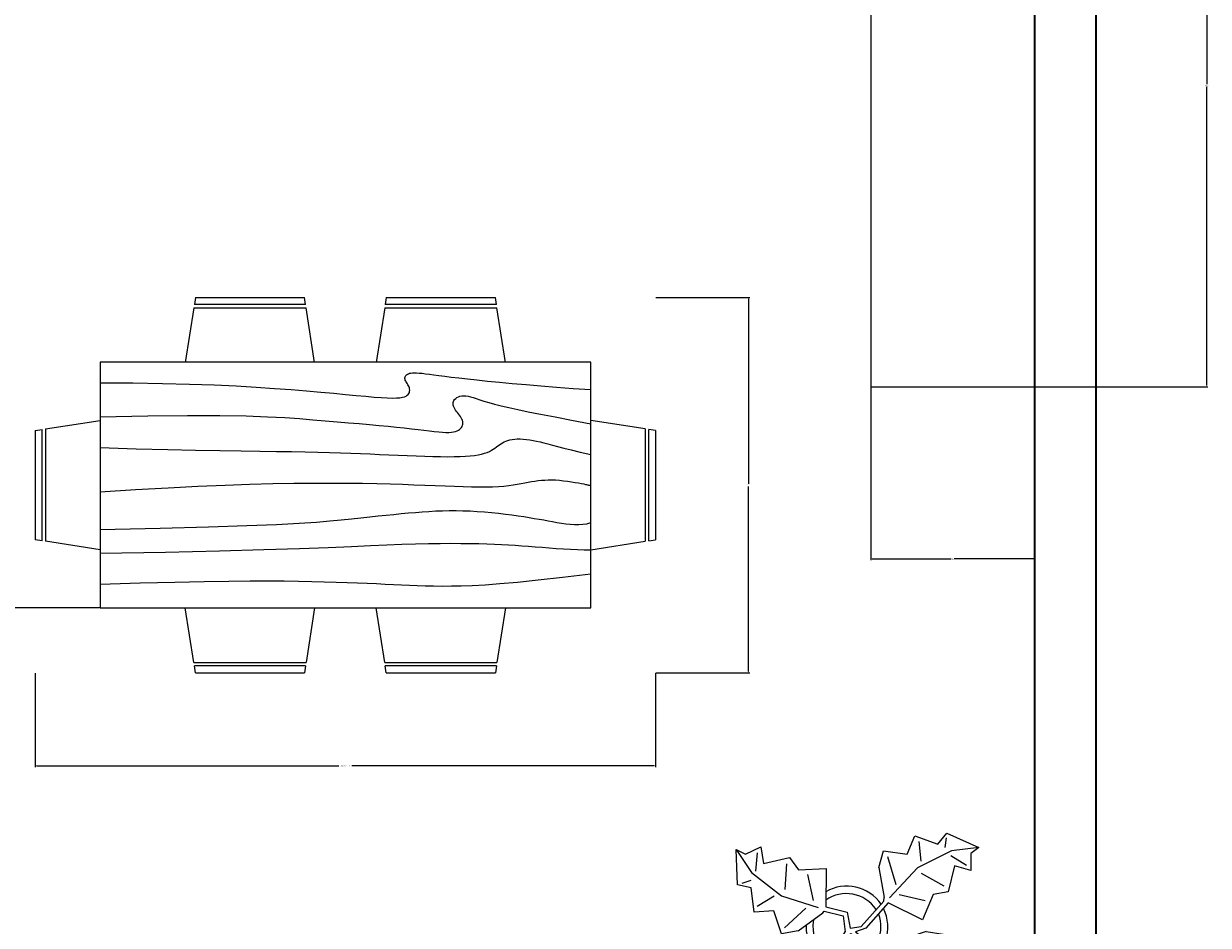
# Model space of a CAD drawing. Units: inches. Extents: x -1 to 436, y -13 to 497.
# Tile 3 of 4: x 227 to 400, y 183 to 315. Entities that reach past the tile are written whole.
import ezdxf

# ---------------------------------------------------------------- set-up
doc = ezdxf.new("R2010")
doc.units = ezdxf.units.IN
for name, color, linetype, lineweight in [('A-ANNO-DIMS', 2, 'Continuous', 18), ('A-FLOR-CASE', 8, 'Continuous', 25), ('A-FURN', 8, 'Continuous', 18), ('A-PLNT', 3, 'Continuous', 13), ('A-WALL', 7, 'Continuous', 35)]:
    doc.layers.add(name, color=color, linetype=linetype, lineweight=lineweight)
doc.styles.get("Standard").update_dxf_attribs({"font": 'arial.ttf'})
doc.dimstyles.get("Standard").update_dxf_attribs({"dimtxt": 0.18, "dimasz": 0.18, "dimexe": 0.18, "dimexo": 0.0625, "dimgap": 0.09, "dimtad": 0, "dimtih": 1, "dimtoh": 1, "dimdec": 4, "dimzin": 0, "dimdsep": 46, "dimtxsty": 'Standard', "dimcen": 0.09, "dimadec": 0, "dimazin": 0, "dimtfac": 1, "dimtdec": 4, "dimtofl": 0, "dimtmove": 0, "dimatfit": 3, "dimfxl": 1, "dimtolj": 1, "dimtzin": 0, "dimarcsym": 0})

# ---------------------------------------------------------------- blocks, each defined once
blk = doc.blocks.new('Dining Set - 36 x 72 in.')
for p, q in [((-22, 27.5), (-22.1562, 26.50042)), ((-5.8416, 26.5), (-22.1534, 26.5)), ((-22, 27.5), (-6, 27.5)), ((-5.8437, 26.49966), (-6, 27.5)), ((6, 27.5), (5.8438, 26.50042)), ((22.1584, 26.5), (5.8466, 26.5)), ((6, 27.5), (22, 27.5)), ((22.1563, 26.49966), (22, 27.5)), ((-22.2343, 26.00059), (-23.4847, 17.99762)), ((-22.2304, 26), (-5.7608, 26)), ((-4.5152, 17.99762), (-5.7655, 25.99926)), ((5.7657, 26.00059), (4.5153, 17.99762)), ((5.7696, 26), (22.2392, 26)), ((23.4848, 17.99762), (22.2345, 25.99926)), ((36, 18), (-36, 18)), ((-36, 18), (-36, -18)), ((36, -18), (36, 18)), ((-44.0006, 8.23428), (-35.9976, 9.48474)), ((44.0006, 8.23428), (35.9976, 9.48474)), ((-45.5, 8), (-44.5004, 8.15617)), ((-45.5, 8), (-45.5, -8)), ((-44.5, -8.15843), (-44.5, 8.15338)), ((-44, 8.23041), (-44, -8.23915)), ((44, 8.23041), (44, -8.23915)), ((44.5, -8.15843), (44.5, 8.15338)), ((45.5, 8), (44.5005, 8.15617)), ((45.5, 8), (45.5, -8)), ((-44.4997, -8.15631), (-45.5, -8)), ((-35.9976, -9.48476), (-43.9993, -8.2345)), ((35.9976, -9.48476), (43.9993, -8.2345)), ((44.4997, -8.15631), (45.5, -8)), ((-36, -18), (36, -18)), ((-22.2343, -26.0006), (-23.4847, -17.99762)), ((-4.5152, -17.99762), (-5.7655, -25.99928)), ((5.7657, -26.0006), (4.5153, -17.99762)), ((23.4848, -17.99762), (22.2345, -25.99928)), ((-22.2304, -26), (-5.7608, -26)), ((5.7696, -26), (22.2392, -26)), ((-22, -27.5), (-22.1562, -26.50044)), ((-5.8416, -26.5), (-22.1534, -26.5)), ((-22, -27.5), (-6, -27.5)), ((-5.8437, -26.49967), (-6, -27.5)), ((6, -27.5), (5.8438, -26.50044)), ((22.1584, -26.5), (5.8466, -26.5)), ((6, -27.5), (22, -27.5)), ((22.1563, -26.49967), (22, -27.5))]:
    blk.add_line(p, q)
for points in [[(-36, 15), (-31.1772, 14.97754), (-26.8079, 14.91406), (-22.8538, 14.81543), (-19.276, 14.6875), (-16.0362, 14.53613), (-13.0957, 14.36718), (-10.4159, 14.18652), (-7.9583, 14), (-5.6904, 13.81315), (-3.6035, 13.63021), (-1.6954, 13.45508), (0.0365, 13.29166), (1.5945, 13.14388), (2.9811, 13.01562), (4.1988, 12.9108), (5.25, 12.83333), (6.1393, 12.78613), (6.8802, 12.76823), (7.4883, 12.77767), (7.9792, 12.8125), (8.3685, 12.87077), (8.6719, 12.95052), (8.9049, 13.0498), (9.0833, 13.16666), (9.2205, 13.29899), (9.3216, 13.44401), (9.3895, 13.59879), (9.4271, 13.76041), (9.4373, 13.92594), (9.4232, 14.09245), (9.3875, 14.257), (9.3333, 14.41666), (9.2638, 14.56917), (9.1836, 14.71484), (9.0975, 14.85465), (9.0104, 14.98958), (8.9272, 15.1206), (8.8529, 15.2487), (8.7922, 15.37483), (8.75, 15.5), (8.7305, 15.62467), (8.7344, 15.74739), (8.7617, 15.86621), (8.8125, 15.97916), (8.8867, 16.08431), (8.9844, 16.17968), (9.1055, 16.26334), (9.25, 16.33333), (9.4189, 16.38802), (9.6172, 16.42708), (9.8506, 16.45052), (10.125, 16.45833), (10.4463, 16.45052), (10.8203, 16.42708), (11.2529, 16.38802), (11.75, 16.33333), (12.3184, 16.26318), (12.9694, 16.17838), (13.7151, 16.07991), (14.5677, 15.96875), (15.5395, 15.84586), (16.6426, 15.71224), (17.8893, 15.56884), (19.2917, 15.41666), (20.859, 15.25667), (22.5879, 15.08984), (24.4721, 14.91715), (26.5052, 14.73958), (28.6809, 14.5581), (30.9929, 14.3737), (33.4347, 14.18733), (36, 14)], [(-36, 10), (-28.9766, 10.14274), (-23.1725, 10.20442), (-18.4241, 10.19775), (-14.5677, 10.13541), (-11.4399, 10.03011), (-8.877, 9.89453), (-6.7154, 9.74137), (-4.7917, 9.58333), (-2.9698, 9.43082), (-1.2246, 9.28515), (0.4415, 9.14534), (2.026, 9.01041), (3.5266, 8.87939), (4.9408, 8.7513), (6.266, 8.62516), (7.5, 8.5), (8.6411, 8.37549), (9.6914, 8.2539), (10.6538, 8.13818), (11.5312, 8.03125), (12.3267, 7.93603), (13.043, 7.85547), (13.6831, 7.79248), (14.25, 7.75), (14.7471, 7.7303), (15.1797, 7.73307), (15.5537, 7.75732), (15.875, 7.80208), (16.1494, 7.86637), (16.3828, 7.94922), (16.5811, 8.04964), (16.75, 8.16666), (16.8944, 8.29915), (17.0143, 8.44531), (17.1089, 8.60319), (17.1771, 8.77083), (17.218, 8.94629), (17.2305, 9.1276), (17.2137, 9.31282), (17.1667, 9.5), (17.0895, 9.6875), (16.987, 9.875), (16.8649, 10.0625), (16.7292, 10.25), (16.5856, 10.4375), (16.4401, 10.625), (16.2985, 10.8125), (16.1667, 11), (16.05, 11.18733), (15.9518, 11.3737), (15.8752, 11.5581), (15.8229, 11.73958), (15.798, 11.91715), (15.8034, 12.08984), (15.842, 12.25667), (15.9167, 12.41666), (16.0295, 12.56836), (16.1784, 12.70833), (16.3605, 12.83268), (16.5729, 12.9375), (16.8127, 13.01888), (17.0768, 13.07291), (17.3625, 13.0957), (17.6667, 13.08333), (17.9894, 13.03312), (18.3418, 12.94726), (18.7382, 12.82918), (19.1927, 12.68229), (19.7195, 12.51001), (20.3327, 12.31575), (21.0465, 12.10294), (21.875, 11.875), (22.8357, 11.63354), (23.959, 11.37304), (25.2786, 11.08618), (26.8282, 10.76562), (28.6414, 10.40405), (30.752, 9.99414), (33.1936, 9.52856), (36, 9)], [(-36, 5.5), (-30.7157, 5.3348), (-26.069, 5.20963), (-21.9946, 5.11767), (-18.4271, 5.05208), (-15.3009, 5.00602), (-12.5508, 4.97265), (-10.1112, 4.94515), (-7.9167, 4.91666), (-5.909, 4.88167), (-4.0586, 4.83984), (-2.3429, 4.79215), (-0.7396, 4.73958), (0.7739, 4.6831), (2.22, 4.6237), (3.6213, 4.56233), (5, 4.5), (6.373, 4.43782), (7.7344, 4.3776), (9.0723, 4.32129), (10.375, 4.27083), (11.6309, 4.22819), (12.8281, 4.19531), (13.9551, 4.17415), (15, 4.16666), (15.954, 4.17448), (16.819, 4.19791), (17.6001, 4.23698), (18.3021, 4.29166), (18.9299, 4.36198), (19.4883, 4.44791), (19.9823, 4.54948), (20.4167, 4.66666), (20.7969, 4.79899), (21.1302, 4.94401), (21.4245, 5.09879), (21.6875, 5.26041), (21.9271, 5.42594), (22.1511, 5.59245), (22.3672, 5.757), (22.5834, 5.91666), (22.8065, 6.06868), (23.0404, 6.21093), (23.2879, 6.34147), (23.5521, 6.45833), (23.8358, 6.55957), (24.142, 6.64323), (24.4735, 6.70735), (24.8334, 6.75), (25.2235, 6.76969), (25.642, 6.76692), (26.0858, 6.74267), (26.5521, 6.69791), (27.0379, 6.63362), (27.5404, 6.55078), (28.0565, 6.45036), (28.5834, 6.33333), (29.1242, 6.19987), (29.7071, 6.04687), (30.3661, 5.87044), (31.1354, 5.66666), (32.0493, 5.43164), (33.142, 5.16146), (34.4475, 4.85221), (36, 4.5)], [(-36, -1), (-30.7915, -0.6591), (-26.0195, -0.38216), (-21.6519, -0.16284), (-17.6563, 0.00521), (-14.0005, 0.12833), (-10.6523, 0.21289), (-7.5796, 0.26522), (-4.75, 0.29166), (-2.134, 0.29793), (0.2878, 0.28711), (2.5317, 0.26163), (4.6146, 0.22396), (6.5529, 0.17651), (8.3633, 0.12174), (10.0623, 0.06209), (11.6667, 0), (13.1899, -0.06201), (14.6341, -0.1211), (15.9982, -0.17432), (17.2813, -0.21875), (18.4823, -0.25147), (19.6003, -0.26953), (20.6343, -0.27002), (21.5834, -0.25), (22.4481, -0.20768), (23.2357, -0.14584), (23.9549, -0.06836), (24.6146, 0.02083), (25.2235, 0.11784), (25.7904, 0.21875), (26.3241, 0.31966), (26.8334, 0.41666), (27.3265, 0.50618), (27.8099, 0.58593), (28.2894, 0.65397), (28.7709, 0.70833), (29.2601, 0.74707), (29.763, 0.76823), (30.2855, 0.76985), (30.8334, 0.75), (31.4088, 0.70784), (31.9994, 0.64713), (32.589, 0.57275), (33.1615, 0.48958), (33.7008, 0.4025), (34.1908, 0.3164), (34.6153, 0.23616), (34.9584, 0.16666), (35.2099, 0.11165), (35.3848, 0.07031), (35.504, 0.04069), (35.5886, 0.02083), (35.6594, 0.00879), (35.7377, 0.0026), (35.8442, 0.00032), (36, 0)], [(-36, -6.5), (-27.1843, -6.31267), (-20.084, -6.1263), (-14.469, -5.9419), (-10.1094, -5.76042), (-6.7752, -5.58285), (-4.2363, -5.41016), (-2.2629, -5.24333), (-0.625, -5.08334), (0.8708, -4.93099), (2.2715, -4.78646), (3.5872, -4.64974), (4.8281, -4.52084), (6.0046, -4.39974), (7.127, -4.28646), (8.2053, -4.18099), (9.25, -4.08334), (10.2705, -3.99382), (11.2734, -3.91407), (12.2647, -3.84603), (13.25, -3.79167), (14.2354, -3.75293), (15.2266, -3.73177), (16.2295, -3.73015), (17.25, -3.75), (18.2912, -3.79248), (19.3451, -3.85547), (20.4009, -3.93604), (21.4479, -4.03125), (22.4754, -4.13819), (23.4727, -4.25391), (24.4289, -4.37549), (25.3334, -4.5), (26.1785, -4.62492), (26.9694, -4.74935), (27.7145, -4.87281), (28.4219, -4.99479), (29.1, -5.11483), (29.7572, -5.23242), (30.4016, -5.34709), (31.0417, -5.45834), (31.6837, -5.56437), (32.3262, -5.65821), (32.9658, -5.73153), (33.599, -5.77604), (34.2224, -5.78345), (34.8327, -5.74545), (35.4264, -5.65373), (36, -5.5)], [(-36, -10), (-26.4022, -9.81299), (-18.4675, -9.62891), (-11.9839, -9.45069), (-6.7396, -9.28125), (-2.5226, -9.12354), (0.8789, -8.98047), (3.6769, -8.85498), (6.0833, -8.75), (8.2767, -8.66765), (10.3021, -8.60677), (12.1712, -8.56543), (13.8958, -8.54167), (15.4876, -8.53353), (16.9583, -8.53907), (18.3197, -8.55632), (19.5834, -8.58334), (20.7616, -8.61841), (21.8685, -8.66081), (22.9188, -8.71004), (23.9271, -8.76563), (24.9081, -8.82707), (25.8763, -8.89388), (26.8465, -8.96558), (27.8334, -9.04167), (28.8474, -9.12118), (29.8828, -9.20117), (30.93, -9.27824), (31.9792, -9.34896), (33.0205, -9.40991), (34.0443, -9.45768), (35.0407, -9.48885), (36, -9.5)], [(-36, -14.5), (-30.0881, -14.33513), (-25.0332, -14.21224), (-20.7312, -14.12647), (-17.0781, -14.07292), (-13.97, -14.04671), (-11.3027, -14.04297), (-8.9724, -14.05681), (-6.875, -14.08334), (-4.9224, -14.11833), (-3.0905, -14.16016), (-1.3709, -14.20785), (0.2448, -14.26042), (1.7647, -14.3169), (3.1973, -14.3763), (4.5507, -14.43767), (5.8333, -14.5), (7.0554, -14.5621), (8.235, -14.62175), (9.3922, -14.67652), (10.5469, -14.72396), (11.7192, -14.76164), (12.929, -14.78711), (14.1965, -14.79794), (15.5417, -14.79167), (16.9933, -14.76424), (18.6152, -14.70508), (20.4804, -14.60197), (22.6615, -14.44271), (25.2312, -14.21509), (28.2624, -13.9069), (31.8277, -13.50594), (36, -13)]]:
    blk.add_lwpolyline(points)
blk = doc.blocks.new('Plant - Rubber or Philodendron')
for p, q in [((13.3837, 12.301), (14.68, 13.9039)), ((14.68, 13.9039), (19.3848, 11.8146)), ((8.8871, 10.7908), (9.9809, 13.4933)), ((9.9809, 13.4933), (13.3837, 12.301)), ((10.5828, 12.6946), (10.8893, 9.7953)), ((14.5816, 13.2037), (14.3848, 11.8033)), ((-16.2005, 11.4774), (-13.9899, 8.1064)), ((-16.2005, 11.4774), (-14.8639, 10.7964)), ((-16.0159, 6.3329), (-16.2005, 11.4774)), ((-14.8639, 10.7964), (-12.6195, 11.8975)), ((-13.3174, 8.325), (-13.0735, 11.0065)), ((-12.6195, 11.8975), (-12.1909, 9.4345)), ((4.6914, 8.8812), (5.3859, 11.2828)), ((5.3859, 11.2828), (8.8871, 10.7908)), ((5.9878, 10.4842), (7.1971, 6.3869)), ((15.3859, 11.3055), (10.3916, 8.7942)), ((15.2875, 10.6053), (17.5907, 9.2105)), ((19.3848, 11.8146), (15.3859, 11.3055)), ((19.3848, 11.8146), (18.1868, 10.9119)), ((18.1868, 10.9119), (18.1925, 8.4119)), ((-12.1909, 9.4345), (-8.3829, 10.3)), ((-8.8369, 9.409), (-9.0894, 5.6095)), ((-8.3829, 10.3), (-7.0549, 8.501)), ((-7.0549, 8.501), (-3.0284, 8.6941)), ((-3.0284, 8.6941), (-3.0709, 3.1041)), ((4.6914, 8.8812), (5.5014, 4.4831)), ((10.3916, 8.7942), (6.2847, 4.4028)), ((15.7909, 9.1065), (14.8995, 5.3044)), ((18.1925, 8.4119), (15.7909, 9.1065)), ((-15.3434, 6.5514), (-13.9984, 6.9884)), ((-13.9899, 8.1064), (-9.5434, 4.7185)), ((-4.8529, 4.012), (-5.7184, 7.82)), ((14.2977, 6.1031), (10.9934, 7.9956)), ((-14.0069, 5.8704), (-16.0159, 6.3329)), ((-13.5868, 2.2894), (-14.0069, 5.8704)), ((14.8995, 5.3044), (12.7005, 4.8994)), ((-13.1329, 3.1804), (-10.6614, 4.727)), ((-9.5434, 4.7185), (-4.1917, 2.9888)), ((2.1141, 0.2298), (5.4346, 3.9146)), ((6.1032, 3.6844), (2.8262, -0.031)), ((5.4346, 3.9146), (5.5014, 4.4831)), ((11.1089, 1.1958), (6.1032, 3.6844)), ((7.7005, 4.8881), (11.5025, 3.9967)), ((12.7005, 4.8994), (11.1089, 1.1958)), ((-10.6784, 2.491), (-13.5868, 2.2894)), ((-9.5858, -0.8715), (-10.6784, 2.491)), ((-9.1318, 0.0195), (-5.9793, 2.9025)), ((-7.1228, -0.443), (-3.5248, 2.2131)), ((-3.5248, 2.2131), (-3.3011, 2.4355)), ((-3.3011, 2.4355), (-0.5306, 1.7947)), ((-3.0709, 3.1041), (0.0797, 2.3163)), ((-0.5306, 1.7947), (-0.2255, -0.5527)), ((-0.5306, 1.7947), (-0.5306, 1.7947)), ((0.0797, 2.3163), (0.4866, -0.031)), ((0.4866, -0.031), (2.1141, 0.2298)), ((-7.1228, -0.443), (-9.5858, -0.8715)), ((-2.019, -3.6148), (-0.2255, -0.5527)), ((-0.9375, -3.1608), (0.5883, -0.8135)), ((0.5883, -0.8135), (2.2447, -2.0916)), ((2.8262, -0.031), (1.3003, -0.5527)), ((1.3003, -0.5527), (2.4193, -1.4655)), ((2.4193, -1.4655), (6.895, -2.1175)), ((11.6605, -0.5413), (6.895, -2.1175)), ((11.6605, -0.5413), (14.1354, -0.8948)), ((14.1354, -0.8948), (14.1354, -4.4304)), ((-4.0579, -6.2781), (-0.9375, -3.1608)), ((2.2447, -2.0916), (6.7108, -2.6626)), ((4.943, -7.9659), (6.7108, -2.6626)), ((12.3677, -6.1981), (7.219, -2.6772)), ((8.3544, -2.7453), (13.1973, -2.1704)), ((-11.3237, -7.2629), (-9.7321, -3.5593)), ((-9.7321, -3.5593), (-4.7264, -6.0479)), ((-2.019, -3.6148), (-4.7264, -6.0479)), ((8.125, -4.0768), (7.7715, -7.9659)), ((14.1354, -4.4304), (16.9638, -5.1375)), ((16.9638, -5.1375), (16.2567, -8.673)), ((-6.3237, -7.2516), (-10.1257, -6.3602)), ((-9.0148, -11.1577), (-4.9047, -6.8122)), ((-4.1246, -6.8466), (-4.0579, -6.2781)), ((-3.3146, -11.2447), (-4.1246, -6.8466)), ((10.2463, -10.4408), (11.6605, -6.9053)), ((15.5496, -10.7943), (12.3677, -6.1981)), ((16.2567, -5.8446), (13.4283, -6.5517)), ((-14.4141, -11.4699), (-13.5228, -7.6679)), ((-13.5228, -7.6679), (-11.3237, -7.2629)), ((-12.921, -8.4665), (-9.6166, -10.359)), ((8.8321, -9.0266), (4.943, -7.9659)), ((16.2567, -8.673), (18.0245, -9.7337)), ((-4.611, -12.8477), (-5.8203, -8.7504)), ((9.5392, -11.1479), (8.8321, -9.0266)), ((17.3174, -9.7337), (15.9032, -9.7337)), ((18.0245, -9.7337), (16.6103, -14.6834)), ((-16.8157, -10.7754), (-14.4141, -11.4699)), ((-16.8101, -13.2754), (-16.8157, -10.7754)), ((-13.9107, -12.9688), (-16.2139, -11.574)), ((-14.0091, -13.669), (-9.0148, -11.1577)), ((-9.206, -15.0581), (-9.5126, -12.1588)), ((-3.3146, -11.2447), (-4.0092, -13.6463)), ((13.4283, -11.5015), (9.5392, -11.1479)), ((13.0748, -13.9763), (13.4283, -11.5015)), ((14.8425, -10.7943), (13.7819, -13.2692)), ((16.6103, -14.6834), (15.5496, -10.7943)), ((-18.008, -14.1781), (-16.8101, -13.2754)), ((-18.008, -14.1781), (-14.0091, -13.669)), ((-7.5103, -13.1543), (-8.6042, -15.8568)), ((-4.0092, -13.6463), (-7.5103, -13.1543)), ((15.5496, -13.6228), (13.0748, -13.9763)), ((16.6103, -14.6834), (15.5496, -13.6228)), ((-13.3032, -16.2674), (-18.008, -14.1781)), ((-12.0069, -14.6645), (-13.3032, -16.2674)), ((-13.2048, -15.5672), (-13.008, -14.1668)), ((-8.6042, -15.8568), (-12.0069, -14.6645))]:
    blk.add_line(p, q)
for centre, radius, start, end in [((0, 0), 6.1275, 34.37569, 120.1028), ((-0.0601, -0.2075), 5.2461, 33.82192, 124.9414), ((-0.2664, 0.1682), 5.2775, 338.4094, 20.03007), ((-0.098, 0.1364), 6.1288, 341.2017, 26.09184), ((0.0308, 0.1664), 6, 178.6147, 235.1169), ((0.0308, 0.1664), 5, 168.1647, 238.6725), ((-0.0234, 0.3825), 6.1492, 242.5812, 331.2714), ((-0.1102, 0.4886), 5.2883, 247.3711, 327.472)]:
    blk.add_arc(centre, radius, start, end)
blk = doc.blocks.new('*D18')
at = {"layer": 'A-ANNO-DIMS', "color": 0, "lineweight": -2, "transparency": 16777216}
for p, q in [((228.39, 219.95), (228.39, 206.18)), ((319.39, 219.95), (319.39, 206.18)), ((228.57, 206.36), (272.94, 206.36)), ((319.21, 206.36), (274.85, 206.36))]:
    blk.add_line(p, q, dxfattribs=at)
at = {"layer": 'A-ANNO-DIMS', "color": 0, "transparency": 16777216}
for points in [[(228.57, 206.39), (228.57, 206.33), (228.39, 206.36)], [(319.21, 206.39), (319.21, 206.33), (319.39, 206.36)]]:
    blk.add_solid(points, dxfattribs=at)
at = {"layer": 'Defpoints', "color": 0, "transparency": 16777216}
for p in [(228.39, 220.01), (319.39, 220.01), (319.39, 206.36)]:
    blk.add_point(p, dxfattribs=at)
at = {"layer": 'A-ANNO-DIMS', "color": 0, "transparency": 16777216, "insert": (273.89, 206.36), "char_height": 0.18, "attachment_point": 5}
blk.add_mtext('\\A1;DINING SET 91', dxfattribs=at)
blk = doc.blocks.new('*D19')
at = {"layer": 'A-ANNO-DIMS', "color": 0, "lineweight": -2, "transparency": 16777216}
for p, q in [((319.46, 275.01), (333.22, 275.01)), ((333.04, 274.83), (333.04, 247.69)), ((333.04, 220.19), (333.04, 247.33)), ((319.46, 220.01), (333.22, 220.01))]:
    blk.add_line(p, q, dxfattribs=at)
at = {"layer": 'A-ANNO-DIMS', "color": 0, "transparency": 16777216}
for points in [[(333.01, 274.83), (333.07, 274.83), (333.04, 275.01)], [(333.01, 220.19), (333.07, 220.19), (333.04, 220.01)]]:
    blk.add_solid(points, dxfattribs=at)
at = {"layer": 'Defpoints', "color": 0, "transparency": 16777216}
for p in [(319.39, 275.01), (333.04, 275.01), (319.39, 220.01)]:
    blk.add_point(p, dxfattribs=at)
at = {"layer": 'A-ANNO-DIMS', "color": 0, "transparency": 16777216, "insert": (333.04, 247.51), "char_height": 0.18, "attachment_point": 5}
blk.add_mtext('\\A1;55', dxfattribs=at)
blk = doc.blocks.new('*D42')
at = {"layer": 'A-ANNO-DIMS', "color": 0, "lineweight": -2, "transparency": 16777216}
for p, q in [((375.06, 350.24), (400.43, 350.24)), ((400.25, 350.06), (400.25, 306.27)), ((400.25, 262.12), (400.25, 305.91)), ((375.06, 261.94), (400.43, 261.94))]:
    blk.add_line(p, q, dxfattribs=at)
at = {"layer": 'A-ANNO-DIMS', "color": 0, "transparency": 16777216}
for points in [[(400.22, 350.06), (400.28, 350.06), (400.25, 350.24)], [(400.22, 262.12), (400.28, 262.12), (400.25, 261.94)]]:
    blk.add_solid(points, dxfattribs=at)
at = {"layer": 'Defpoints', "color": 0, "transparency": 16777216}
for p in [(375, 350.24), (375, 261.94), (400.25, 261.94)]:
    blk.add_point(p, dxfattribs=at)
at = {"layer": 'A-ANNO-DIMS', "color": 0, "transparency": 16777216, "insert": (400.25, 306.09), "char_height": 0.18, "attachment_point": 5}
blk.add_mtext('\\A1;88.3', dxfattribs=at)
blk = doc.blocks.new('*D43')
at = {"layer": 'A-ANNO-DIMS', "color": 0, "lineweight": -2, "transparency": 16777216}
for p, q in [((351, 261.88), (351, 236.51)), ((375, 261.88), (375, 236.51)), ((351.18, 236.69), (362.78, 236.69)), ((374.82, 236.69), (363.22, 236.69))]:
    blk.add_line(p, q, dxfattribs=at)
at = {"layer": 'A-ANNO-DIMS', "color": 0, "transparency": 16777216}
for points in [[(351.18, 236.72), (351.18, 236.66), (351, 236.69)], [(374.82, 236.72), (374.82, 236.66), (375, 236.69)]]:
    blk.add_solid(points, dxfattribs=at)
at = {"layer": 'Defpoints', "color": 0, "transparency": 16777216}
for p in [(351, 261.94), (375, 261.94), (351, 236.69)]:
    blk.add_point(p, dxfattribs=at)
at = {"layer": 'A-ANNO-DIMS', "color": 0, "transparency": 16777216, "insert": (363, 236.69), "char_height": 0.18, "attachment_point": 5}
blk.add_mtext('\\A1;24', dxfattribs=at)
blk = doc.blocks.new('*D72')
at = {"layer": 'A-ANNO-DIMS', "color": 0, "lineweight": -2, "transparency": 16777216}
for p, q in [((237.83, 229.51), (212.46, 229.53)), ((212.64, 229.35), (212.61, 192.7)), ((212.58, 155.69), (212.61, 192.34)), ((237.77, 155.49), (212.4, 155.51))]:
    blk.add_line(p, q, dxfattribs=at)
at = {"layer": 'A-ANNO-DIMS', "color": 0, "transparency": 16777216}
for points in [[(212.61, 229.35), (212.67, 229.35), (212.64, 229.53)], [(212.55, 155.69), (212.61, 155.69), (212.58, 155.51)]]:
    blk.add_solid(points, dxfattribs=at)
at = {"layer": 'Defpoints', "color": 0, "transparency": 16777216}
for p in [(212.64, 229.53), (237.89, 229.51), (237.83, 155.49)]:
    blk.add_point(p, dxfattribs=at)
at = {"layer": 'A-ANNO-DIMS', "color": 0, "transparency": 16777216, "insert": (212.61, 192.52), "char_height": 0.18, "attachment_point": 5}
blk.add_mtext('\\A1;74.03', dxfattribs=at)

msp = doc.modelspace()

# ---------------------------------------------------------------- linework, layer by layer
at = {"layer": 'A-FLOR-CASE'}
for p, q in [((351, 390.5331), (351, 261.9384)), ((351, 261.9384), (375, 261.9384))]:
    msp.add_line(p, q, dxfattribs=at)
at = {"layer": 'A-WALL'}
for p, q in [((384, 471.5331), (384, 185.0331)), ((384, 471.5331), (384, 12.5331)), ((375, 390.5331), (375, 21.5331))]:
    msp.add_line(p, q, dxfattribs=at)

# ---------------------------------------------------------------- block references
at = {"layer": 'A-FURN'}
msp.add_blockref('Dining Set - 36 x 72 in.', (273.8948, 247.5117), dxfattribs=at)
at = {"layer": 'A-PLNT'}
msp.add_blockref('Plant - Rubber or Philodendron', (347.4393, 182.5896), dxfattribs=at)

# ---------------------------------------------------------------- dimensions: what is measured, and where the dimension line sits
at = {"layer": 'A-ANNO-DIMS'}
for base, p1, p2, angle, override, picture, middle in [((400.25, 261.9384), (375, 350.238), (375, 261.9384), 270, {"dimdec": 1, "dimlfac": 1, "dimrnd": 0, "dimzin": 0, "dimdsep": 46, "dimlunit": 2}, '*D42', (400.25, 306.0882)), ((333.0448, 275.0117), (319.3948, 220.0117), (319.3948, 275.0117), 90, {"dimdec": 0, "dimlfac": 1, "dimrnd": 0, "dimzin": 0, "dimdsep": 46, "dimlunit": 2}, '*D19', (333.0448, 247.5117)), ((351, 236.6884), (375, 261.9384), (351, 261.9384), 180, {"dimdec": 0, "dimlfac": 1, "dimrnd": 0, "dimzin": 0, "dimdsep": 46, "dimlunit": 2}, '*D43', (363, 236.6884)), ((212.6448, 229.5338), (237.8302, 155.4864), (237.8948, 229.5117), 89.949986, {"dimdec": 2, "dimlfac": 1, "dimrnd": 0, "dimzin": 0, "dimdsep": 46, "dimlunit": 2}, '*D72', (212.6125, 192.5211))]:
    dim = msp.add_linear_dim(base=base, p1=p1, p2=p2, angle=angle, dimstyle='Standard', override=override, dxfattribs=at)
    dim.commit()
    dim.dimension.update_dxf_attribs({"geometry": picture, "text_midpoint": middle})
dim = msp.add_linear_dim(base=(319.3948, 206.3617), p1=(228.3948, 220.0117), p2=(319.3948, 220.0117), text='DINING SET <>', dimstyle='Standard', override={"dimdec": 0, "dimlfac": 1, "dimrnd": 0, "dimzin": 0, "dimdsep": 46, "dimlunit": 2}, dxfattribs=at)
dim.commit()
dim.dimension.update_dxf_attribs({"geometry": '*D18', "text_midpoint": (273.8948, 206.3617)})

doc.saveas('drawing.dxf')
